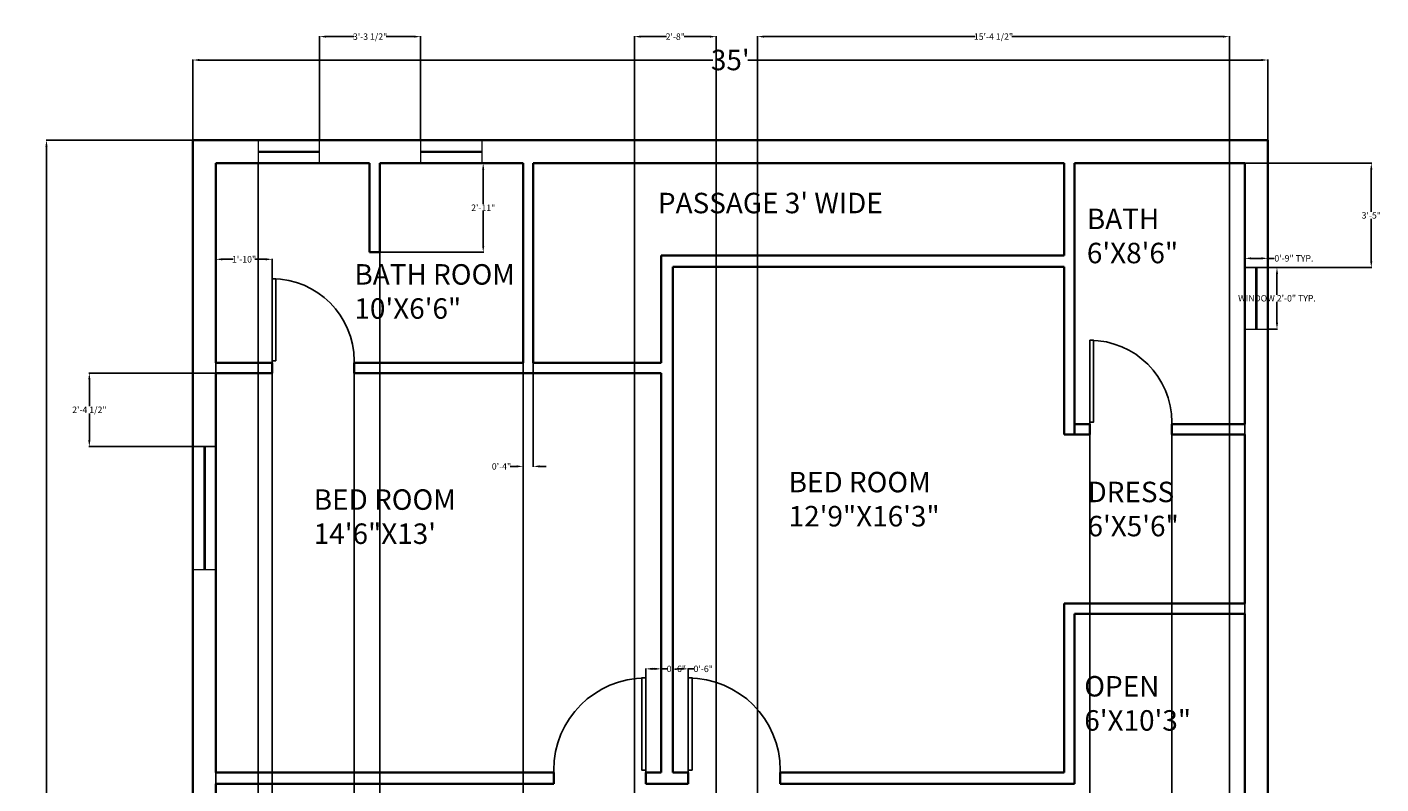
# Model space of a CAD drawing. Units: inches. Extents: x 1737 to 2270, y 2551 to 3419.
# Tile 4 of 4: x 1737 to 2266, y 3124 to 3419. Entities that reach past the tile are written whole.
import ezdxf

# ---------------------------------------------------------------- set-up
doc = ezdxf.new("R2010")
doc.units = ezdxf.units.IN
doc.header["$MEASUREMENT"] = 0
doc.layers.get('0').update_dxf_attribs({"color": 60})
for name, color, linetype, lineweight in [('A-ANNO-DIMS', 2, 'Continuous', 18), ('A-AREA-IDEN', 231, 'Continuous', 18), ('DOOR', 20, 'Continuous', 25), ('WALL', 60, 'Continuous', 35), ('WINDOW', 30, 'Continuous', 18)]:
    doc.layers.add(name, color=color, linetype=linetype, lineweight=lineweight)
doc.styles.get("Standard").update_dxf_attribs({"font": 'arial.ttf'})
doc.dimstyles.get("Standard").update_dxf_attribs({"dimtxt": 2.5, "dimasz": 2.5, "dimexe": 0.18, "dimexo": 0.0625, "dimgap": 0.09, "dimtad": 0, "dimtih": 1, "dimtoh": 1, "dimzin": 0, "dimdsep": 46, "dimlunit": 3, "dimtxsty": 'Standard', "dimcen": 0.09, "dimadec": 0, "dimazin": 0, "dimtfac": 1, "dimtofl": 0, "dimtmove": 0, "dimatfit": 3, "dimfxl": 1, "dimtolj": 1, "dimtzin": 0, "dimarcsym": 0})

# ---------------------------------------------------------------- blocks, each defined once
blk = doc.blocks.new('*U2')
for p, q in [((0, 0), (0, -6)), ((40, 0), (40, -6))]:
    blk.add_line(p, q)
blk.add_lwpolyline([(0, 0), (0, 40), (1.75, 40), (1.75, 0)], close=True)
blk.add_arc((0, 0), 40, 0, 90)
blk = doc.blocks.new('*D5')
at = {"layer": 'A-ANNO-DIMS', "color": 0, "lineweight": -2, "transparency": 16777216}
for p, q in [((1802.15, 3375.16), (1744.83, 3375.16)), ((1745.01, 3372.66), (1745.01, 2989.33)), ((1745.01, 2597.66), (1745.01, 2980.98)), ((1802.15, 2595.16), (1744.83, 2595.16))]:
    blk.add_line(p, q, dxfattribs=at)
at = {"layer": 'A-ANNO-DIMS', "color": 0, "transparency": 16777216}
for points in [[(1744.59, 3372.66), (1745.42, 3372.66), (1745.01, 3375.16)], [(1744.59, 2597.66), (1745.42, 2597.66), (1745.01, 2595.16)]]:
    blk.add_solid(points, dxfattribs=at)
at = {"layer": 'Defpoints', "color": 0, "transparency": 16777216}
for p in [(1802.21, 3375.16), (1745.01, 2595.16), (1802.21, 2595.16)]:
    blk.add_point(p, dxfattribs=at)
at = {"layer": 'A-ANNO-DIMS', "color": 0, "transparency": 16777216, "insert": (1745.01, 2985.16), "char_height": 8, "attachment_point": 5}
blk.add_mtext("\\A1;65'", dxfattribs=at)
blk = doc.blocks.new('*D6')
at = {"layer": 'A-ANNO-DIMS', "color": 0, "lineweight": -2, "transparency": 16777216}
for p, q in [((1802.21, 3375.22), (1802.21, 3406.65)), ((1804.71, 3406.47), (2005.33, 3406.47)), ((2219.71, 3406.47), (2019.08, 3406.47)), ((2222.21, 3375.22), (2222.21, 3406.65))]:
    blk.add_line(p, q, dxfattribs=at)
at = {"layer": 'A-ANNO-DIMS', "color": 0, "transparency": 16777216}
for points in [[(1804.71, 3406.88), (1804.71, 3406.05), (1802.21, 3406.47)], [(2219.71, 3406.88), (2219.71, 3406.05), (2222.21, 3406.47)]]:
    blk.add_solid(points, dxfattribs=at)
at = {"layer": 'Defpoints', "color": 0, "transparency": 16777216}
for p in [(2222.21, 3406.47), (1802.21, 3375.16), (2222.21, 3375.16)]:
    blk.add_point(p, dxfattribs=at)
at = {"layer": 'A-ANNO-DIMS', "color": 0, "transparency": 16777216, "insert": (2012.21, 3406.47), "char_height": 8, "attachment_point": 5}
blk.add_mtext("\\A1;35'", dxfattribs=at)
blk = doc.blocks.new('WIN-48IN')
for p, q in [((4.25, 48), (4.25, 0)), ((4.75, 48), (4.75, 0))]:
    blk.add_line(p, q)
blk.add_lwpolyline([(0, 48), (0, 0), (9, 0), (9, 48)], close=True)
blk = doc.blocks.new('WIN-24IN')
for p, q in [((0, 4.75), (24, 4.75)), ((0, 4.25), (24, 4.25))]:
    blk.add_line(p, q)
blk.add_lwpolyline([(0, 0), (24, 0), (24, 9), (0, 9)], close=True)
blk = doc.blocks.new('*D11')
at = {"layer": 'A-ANNO-DIMS', "color": 0, "lineweight": -2, "transparency": 16777216}
for p, q in [((2222.27, 3325.38), (2225.99, 3325.38)), ((2225.81, 3322.88), (2225.81, 3314.76)), ((2225.81, 3303.88), (2225.81, 3311.99)), ((2222.27, 3301.38), (2225.99, 3301.38))]:
    blk.add_line(p, q, dxfattribs=at)
at = {"layer": 'A-ANNO-DIMS', "color": 0, "transparency": 16777216}
for points in [[(2225.39, 3322.88), (2226.23, 3322.88), (2225.81, 3325.38)], [(2225.39, 3303.88), (2226.23, 3303.88), (2225.81, 3301.38)]]:
    blk.add_solid(points, dxfattribs=at)
at = {"layer": 'Defpoints', "color": 0, "transparency": 16777216}
for p in [(2222.21, 3325.38), (2222.21, 3301.38), (2225.81, 3301.38)]:
    blk.add_point(p, dxfattribs=at)
at = {"layer": 'A-ANNO-DIMS', "color": 0, "transparency": 16777216, "insert": (2225.81, 3313.38), "char_height": 2.5, "attachment_point": 5}
blk.add_mtext('\\A1;WINDOW 2\'-0" TYP.', dxfattribs=at)
blk = doc.blocks.new('*D12')
at = {"layer": 'A-ANNO-DIMS', "color": 0, "lineweight": -2, "transparency": 16777216}
for p, q in [((2213.21, 3325.44), (2213.21, 3329.16)), ((2215.71, 3328.98), (2219.71, 3328.98)), ((2222.21, 3325.44), (2222.21, 3329.16)), ((2222.21, 3328.98), (2224.71, 3328.98))]:
    blk.add_line(p, q, dxfattribs=at)
at = {"layer": 'A-ANNO-DIMS', "color": 0, "transparency": 16777216}
for points in [[(2215.71, 3329.39), (2215.71, 3328.56), (2213.21, 3328.98)], [(2219.71, 3329.39), (2219.71, 3328.56), (2222.21, 3328.98)]]:
    blk.add_solid(points, dxfattribs=at)
at = {"layer": 'Defpoints', "color": 0, "transparency": 16777216}
for p in [(2222.21, 3328.98), (2213.21, 3325.38), (2222.21, 3325.38)]:
    blk.add_point(p, dxfattribs=at)
at = {"layer": 'A-ANNO-DIMS', "color": 0, "transparency": 16777216, "insert": (2232.42, 3328.98), "char_height": 2.5, "attachment_point": 5}
blk.add_mtext('\\A1;0\'-9" TYP.', dxfattribs=at)
blk = doc.blocks.new('*D15')
at = {"layer": 'A-ANNO-DIMS', "color": 0, "lineweight": -2, "transparency": 16777216}
for p, q in [((1811.15, 3284.16), (1761.58, 3284.16)), ((1761.76, 3281.66), (1761.76, 3271.2)), ((1761.76, 3257.98), (1761.76, 3268.43)), ((1811.15, 3255.48), (1761.58, 3255.48))]:
    blk.add_line(p, q, dxfattribs=at)
at = {"layer": 'A-ANNO-DIMS', "color": 0, "transparency": 16777216}
for points in [[(1761.34, 3281.66), (1762.18, 3281.66), (1761.76, 3284.16)], [(1761.34, 3257.98), (1762.18, 3257.98), (1761.76, 3255.48)]]:
    blk.add_solid(points, dxfattribs=at)
at = {"layer": 'Defpoints', "color": 0, "transparency": 16777216}
for p in [(1811.21, 3284.16), (1761.76, 3255.48), (1811.21, 3255.48)]:
    blk.add_point(p, dxfattribs=at)
at = {"layer": 'A-ANNO-DIMS', "color": 0, "transparency": 16777216, "insert": (1761.76, 3269.82), "char_height": 2.5, "attachment_point": 5}
blk.add_mtext('\\A1;2\'-4 1/2"', dxfattribs=at)
blk = doc.blocks.new('*D17')
at = {"layer": 'A-ANNO-DIMS', "color": 0, "lineweight": -2, "transparency": 16777216}
for p, q in [((2213.27, 3366.16), (2262.84, 3366.16)), ((2262.66, 3363.66), (2262.66, 3347.13)), ((2262.66, 3327.88), (2262.66, 3344.4)), ((2213.27, 3325.38), (2262.84, 3325.38))]:
    blk.add_line(p, q, dxfattribs=at)
at = {"layer": 'A-ANNO-DIMS', "color": 0, "transparency": 16777216}
for points in [[(2262.24, 3363.66), (2263.08, 3363.66), (2262.66, 3366.16)], [(2262.24, 3327.88), (2263.08, 3327.88), (2262.66, 3325.38)]]:
    blk.add_solid(points, dxfattribs=at)
at = {"layer": 'Defpoints', "color": 0, "transparency": 16777216}
for p in [(2213.21, 3366.16), (2213.21, 3325.38), (2262.66, 3325.38)]:
    blk.add_point(p, dxfattribs=at)
at = {"layer": 'A-ANNO-DIMS', "color": 0, "transparency": 16777216, "insert": (2262.66, 3345.77), "char_height": 2.5, "attachment_point": 5}
blk.add_mtext('\\A1;3\'-5"', dxfattribs=at)
blk = doc.blocks.new('*D18')
at = {"layer": 'A-ANNO-DIMS', "color": 0, "lineweight": -2, "transparency": 16777216}
for p, q in [((1811.21, 3366.1), (1811.21, 2554.53)), ((1827.73, 3366.1), (1827.73, 2554.53)), ((1808.71, 2554.71), (1806.21, 2554.71)), ((1830.23, 2554.71), (1832.73, 2554.71))]:
    blk.add_line(p, q, dxfattribs=at)
at = {"layer": 'A-ANNO-DIMS', "color": 0, "transparency": 16777216}
for points in [[(1808.71, 2555.12), (1808.71, 2554.29), (1811.21, 2554.71)], [(1830.23, 2555.12), (1830.23, 2554.29), (1827.73, 2554.71)]]:
    blk.add_solid(points, dxfattribs=at)
at = {"layer": 'Defpoints', "color": 0, "transparency": 16777216}
for p in [(1811.21, 3366.16), (1827.73, 3366.16), (1827.73, 2554.71)]:
    blk.add_point(p, dxfattribs=at)
at = {"layer": 'A-ANNO-DIMS', "color": 0, "transparency": 16777216, "insert": (1819.47, 2554.71), "char_height": 2.5, "attachment_point": 5}
blk.add_mtext('\\A1;1\'-4 1/2"', dxfattribs=at)
blk = doc.blocks.new('*D19')
at = {"layer": 'A-ANNO-DIMS', "color": 0, "lineweight": -2, "transparency": 16777216}
for p, q in [((1851.73, 3375.22), (1851.73, 3415.79)), ((1854.23, 3415.61), (1865.13, 3415.61)), ((1888.69, 3415.61), (1877.78, 3415.61)), ((1891.19, 3375.22), (1891.19, 3415.79))]:
    blk.add_line(p, q, dxfattribs=at)
at = {"layer": 'A-ANNO-DIMS', "color": 0, "transparency": 16777216}
for points in [[(1854.23, 3416.02), (1854.23, 3415.19), (1851.73, 3415.61)], [(1888.69, 3416.02), (1888.69, 3415.19), (1891.19, 3415.61)]]:
    blk.add_solid(points, dxfattribs=at)
at = {"layer": 'Defpoints', "color": 0, "transparency": 16777216}
for p in [(1891.19, 3415.61), (1851.73, 3375.16), (1891.19, 3375.16)]:
    blk.add_point(p, dxfattribs=at)
at = {"layer": 'A-ANNO-DIMS', "color": 0, "transparency": 16777216, "insert": (1871.46, 3415.61), "char_height": 2.5, "attachment_point": 5}
blk.add_mtext('\\A1;3\'-3 1/2"', dxfattribs=at)
blk = doc.blocks.new('*D20')
at = {"layer": 'A-ANNO-DIMS', "color": 0, "lineweight": -2, "transparency": 16777216}
for p, q in [((2022.87, 2595.22), (2022.87, 3415.79)), ((2025.37, 3415.61), (2107.86, 3415.61)), ((2204.71, 3415.61), (2122.22, 3415.61)), ((2207.21, 2595.22), (2207.21, 3415.79))]:
    blk.add_line(p, q, dxfattribs=at)
at = {"layer": 'A-ANNO-DIMS', "color": 0, "transparency": 16777216}
for points in [[(2025.37, 3416.02), (2025.37, 3415.19), (2022.87, 3415.61)], [(2204.71, 3416.02), (2204.71, 3415.19), (2207.21, 3415.61)]]:
    blk.add_solid(points, dxfattribs=at)
at = {"layer": 'Defpoints', "color": 0, "transparency": 16777216}
for p in [(2207.21, 3415.61), (2022.87, 2595.16), (2207.21, 2595.16)]:
    blk.add_point(p, dxfattribs=at)
at = {"layer": 'A-ANNO-DIMS', "color": 0, "transparency": 16777216, "insert": (2115.04, 3415.61), "char_height": 2.5, "attachment_point": 5}
blk.add_mtext('\\A1;15\'-4 1/2"', dxfattribs=at)
blk = doc.blocks.new('*D24')
at = {"layer": 'A-ANNO-DIMS', "color": 0, "lineweight": -2, "transparency": 16777216}
for p, q in [((1833.21, 3284.1), (1833.21, 2554.53)), ((1865.21, 3284.1), (1865.21, 2554.53)), ((1835.71, 2554.71), (1845.77, 2554.71)), ((1862.71, 2554.71), (1852.64, 2554.71))]:
    blk.add_line(p, q, dxfattribs=at)
at = {"layer": 'A-ANNO-DIMS', "color": 0, "transparency": 16777216}
for points in [[(1835.71, 2555.12), (1835.71, 2554.29), (1833.21, 2554.71)], [(1862.71, 2555.12), (1862.71, 2554.29), (1865.21, 2554.71)]]:
    blk.add_solid(points, dxfattribs=at)
at = {"layer": 'Defpoints', "color": 0, "transparency": 16777216}
for p in [(1833.21, 3284.16), (1865.21, 3284.16), (1865.21, 2554.71)]:
    blk.add_point(p, dxfattribs=at)
at = {"layer": 'A-ANNO-DIMS', "color": 0, "transparency": 16777216, "insert": (1849.21, 2554.71), "char_height": 2.5, "attachment_point": 5}
blk.add_mtext('\\A1;2\'-8"', dxfattribs=at)
blk = doc.blocks.new('*D29')
at = {"layer": 'A-ANNO-DIMS', "color": 0, "lineweight": -2, "transparency": 16777216}
for p, q in [((1974.71, 2758.72), (1974.71, 3415.79)), ((1977.21, 3415.61), (1987.27, 3415.61)), ((2004.21, 3415.61), (1994.14, 3415.61)), ((2006.71, 2758.72), (2006.71, 3415.79))]:
    blk.add_line(p, q, dxfattribs=at)
at = {"layer": 'A-ANNO-DIMS', "color": 0, "transparency": 16777216}
for points in [[(1977.21, 3416.02), (1977.21, 3415.19), (1974.71, 3415.61)], [(2004.21, 3416.02), (2004.21, 3415.19), (2006.71, 3415.61)]]:
    blk.add_solid(points, dxfattribs=at)
at = {"layer": 'Defpoints', "color": 0, "transparency": 16777216}
for p in [(2006.71, 3415.61), (1974.71, 2758.66), (2006.71, 2758.66)]:
    blk.add_point(p, dxfattribs=at)
at = {"layer": 'A-ANNO-DIMS', "color": 0, "transparency": 16777216, "insert": (1990.71, 3415.61), "char_height": 2.5, "attachment_point": 5}
blk.add_mtext('\\A1;2\'-8"', dxfattribs=at)
blk = doc.blocks.new('*D33')
at = {"layer": 'A-ANNO-DIMS', "color": 0, "lineweight": -2, "transparency": 16777216}
for p, q in [((1811.21, 3288.22), (1811.21, 3328.79)), ((1813.71, 3328.61), (1817.94, 3328.61)), ((1830.71, 3328.61), (1826.48, 3328.61)), ((1833.21, 3288.22), (1833.21, 3328.79))]:
    blk.add_line(p, q, dxfattribs=at)
at = {"layer": 'A-ANNO-DIMS', "color": 0, "transparency": 16777216}
for points in [[(1813.71, 3329.02), (1813.71, 3328.19), (1811.21, 3328.61)], [(1830.71, 3329.02), (1830.71, 3328.19), (1833.21, 3328.61)]]:
    blk.add_solid(points, dxfattribs=at)
at = {"layer": 'Defpoints', "color": 0, "transparency": 16777216}
for p in [(1833.21, 3328.61), (1811.21, 3288.16), (1833.21, 3288.16)]:
    blk.add_point(p, dxfattribs=at)
at = {"layer": 'A-ANNO-DIMS', "color": 0, "transparency": 16777216, "insert": (1822.21, 3328.61), "char_height": 2.5, "attachment_point": 5}
blk.add_mtext('\\A1;1\'-10"', dxfattribs=at)
blk = doc.blocks.new('*D36')
at = {"layer": 'A-ANNO-DIMS', "color": 0, "lineweight": -2, "transparency": 16777216}
for p, q in [((2152.71, 3260.1), (2152.71, 2554.53)), ((2184.71, 3260.1), (2184.71, 2554.53)), ((2155.21, 2554.71), (2165.27, 2554.71)), ((2182.21, 2554.71), (2172.14, 2554.71))]:
    blk.add_line(p, q, dxfattribs=at)
at = {"layer": 'A-ANNO-DIMS', "color": 0, "transparency": 16777216}
for points in [[(2155.21, 2555.12), (2155.21, 2554.29), (2152.71, 2554.71)], [(2182.21, 2555.12), (2182.21, 2554.29), (2184.71, 2554.71)]]:
    blk.add_solid(points, dxfattribs=at)
at = {"layer": 'Defpoints', "color": 0, "transparency": 16777216}
for p in [(2152.71, 3260.16), (2184.71, 3260.16), (2184.71, 2554.71)]:
    blk.add_point(p, dxfattribs=at)
at = {"layer": 'A-ANNO-DIMS', "color": 0, "transparency": 16777216, "insert": (2168.71, 2554.71), "char_height": 2.5, "attachment_point": 5}
blk.add_mtext('\\A1;2\'-8"', dxfattribs=at)
blk = doc.blocks.new('*D38')
at = {"layer": 'A-ANNO-DIMS', "color": 0, "lineweight": -2, "transparency": 16777216}
for p, q in [((1875.27, 3366.16), (1915.84, 3366.16)), ((1915.66, 3363.66), (1915.66, 3350.1)), ((1915.66, 3333.86), (1915.66, 3347.41)), ((1875.27, 3331.36), (1915.84, 3331.36))]:
    blk.add_line(p, q, dxfattribs=at)
at = {"layer": 'A-ANNO-DIMS', "color": 0, "transparency": 16777216}
for points in [[(1915.24, 3363.66), (1916.08, 3363.66), (1915.66, 3366.16)], [(1915.24, 3333.86), (1916.08, 3333.86), (1915.66, 3331.36)]]:
    blk.add_solid(points, dxfattribs=at)
at = {"layer": 'Defpoints', "color": 0, "transparency": 16777216}
for p in [(1875.21, 3366.16), (1875.21, 3331.36), (1915.66, 3331.36)]:
    blk.add_point(p, dxfattribs=at)
at = {"layer": 'A-ANNO-DIMS', "color": 0, "transparency": 16777216, "insert": (1915.66, 3348.76), "char_height": 2.5, "attachment_point": 5}
blk.add_mtext('\\A1;2\'-11"', dxfattribs=at)
blk = doc.blocks.new('*D39')
at = {"layer": 'A-ANNO-DIMS', "color": 0, "lineweight": -2, "transparency": 16777216}
for p, q in [((1875.21, 3366.1), (1875.21, 2554.53)), ((1931.21, 3366.1), (1931.21, 2554.53)), ((1877.71, 2554.71), (1899.75, 2554.71)), ((1928.71, 2554.71), (1906.67, 2554.71))]:
    blk.add_line(p, q, dxfattribs=at)
at = {"layer": 'A-ANNO-DIMS', "color": 0, "transparency": 16777216}
for points in [[(1877.71, 2555.12), (1877.71, 2554.29), (1875.21, 2554.71)], [(1928.71, 2555.12), (1928.71, 2554.29), (1931.21, 2554.71)]]:
    blk.add_solid(points, dxfattribs=at)
at = {"layer": 'Defpoints', "color": 0, "transparency": 16777216}
for p in [(1875.21, 3366.16), (1931.21, 3366.16), (1931.21, 2554.71)]:
    blk.add_point(p, dxfattribs=at)
at = {"layer": 'A-ANNO-DIMS', "color": 0, "transparency": 16777216, "insert": (1903.21, 2554.71), "char_height": 2.5, "attachment_point": 5}
blk.add_mtext('\\A1;4\'-8"', dxfattribs=at)
blk = doc.blocks.new('*D40')
at = {"layer": 'A-ANNO-DIMS', "color": 0, "lineweight": -2, "transparency": 16777216}
for p, q in [((1979.21, 3128.22), (1979.21, 3168.79)), ((1985.21, 3128.22), (1985.21, 3168.79)), ((1981.71, 3168.61), (1982.71, 3168.61)), ((1985.21, 3168.61), (1987.71, 3168.61))]:
    blk.add_line(p, q, dxfattribs=at)
at = {"layer": 'A-ANNO-DIMS', "color": 0, "transparency": 16777216}
for points in [[(1981.71, 3169.02), (1981.71, 3168.19), (1979.21, 3168.61)], [(1982.71, 3169.02), (1982.71, 3168.19), (1985.21, 3168.61)]]:
    blk.add_solid(points, dxfattribs=at)
at = {"layer": 'Defpoints', "color": 0, "transparency": 16777216}
for p in [(1985.21, 3168.61), (1979.21, 3128.16), (1985.21, 3128.16)]:
    blk.add_point(p, dxfattribs=at)
at = {"layer": 'A-ANNO-DIMS', "color": 0, "transparency": 16777216, "insert": (1991.12, 3168.61), "char_height": 2.5, "attachment_point": 5}
blk.add_mtext('\\A1;0\'-6"', dxfattribs=at)
blk = doc.blocks.new('*D41')
at = {"layer": 'A-ANNO-DIMS', "color": 0, "lineweight": -2, "transparency": 16777216}
for p, q in [((1989.71, 3128.22), (1989.71, 3168.79)), ((1995.71, 3128.22), (1995.71, 3168.79)), ((1992.21, 3168.61), (1993.21, 3168.61)), ((1995.71, 3168.61), (1998.21, 3168.61))]:
    blk.add_line(p, q, dxfattribs=at)
at = {"layer": 'A-ANNO-DIMS', "color": 0, "transparency": 16777216}
for points in [[(1992.21, 3169.02), (1992.21, 3168.19), (1989.71, 3168.61)], [(1993.21, 3169.02), (1993.21, 3168.19), (1995.71, 3168.61)]]:
    blk.add_solid(points, dxfattribs=at)
at = {"layer": 'Defpoints', "color": 0, "transparency": 16777216}
for p in [(1995.71, 3168.61), (1989.71, 3128.16), (1995.71, 3128.16)]:
    blk.add_point(p, dxfattribs=at)
at = {"layer": 'A-ANNO-DIMS', "color": 0, "transparency": 16777216, "insert": (2001.62, 3168.61), "char_height": 2.5, "attachment_point": 5}
blk.add_mtext('\\A1;0\'-6"', dxfattribs=at)
blk = doc.blocks.new('*D42')
at = {"layer": 'A-ANNO-DIMS', "color": 0, "lineweight": -2, "transparency": 16777216}
for p, q in [((2213.21, 3264.1), (2213.21, 2554.53)), ((2184.71, 3263.5), (2184.71, 2554.53)), ((2187.21, 2554.71), (2192.61, 2554.71)), ((2210.71, 2554.71), (2205.31, 2554.71))]:
    blk.add_line(p, q, dxfattribs=at)
at = {"layer": 'A-ANNO-DIMS', "color": 0, "transparency": 16777216}
for points in [[(2187.21, 2555.12), (2187.21, 2554.29), (2184.71, 2554.71)], [(2210.71, 2555.12), (2210.71, 2554.29), (2213.21, 2554.71)]]:
    blk.add_solid(points, dxfattribs=at)
at = {"layer": 'Defpoints', "color": 0, "transparency": 16777216}
for p in [(2213.21, 3264.16), (2184.71, 3263.56), (2213.21, 2554.71)]:
    blk.add_point(p, dxfattribs=at)
at = {"layer": 'A-ANNO-DIMS', "color": 0, "transparency": 16777216, "insert": (2198.96, 2554.71), "char_height": 2.5, "attachment_point": 5}
blk.add_mtext('\\A1;2\'-4 1/2"', dxfattribs=at)
blk = doc.blocks.new('*D52')
at = {"layer": 'A-ANNO-DIMS', "color": 0, "lineweight": -2, "transparency": 16777216}
for p, q in [((1931.21, 3288.1), (1931.21, 3247.53)), ((1935.21, 3288.1), (1935.21, 3247.53)), ((1928.71, 3247.71), (1926.21, 3247.71)), ((1937.71, 3247.71), (1940.21, 3247.71))]:
    blk.add_line(p, q, dxfattribs=at)
at = {"layer": 'A-ANNO-DIMS', "color": 0, "transparency": 16777216}
for points in [[(1928.71, 3248.12), (1928.71, 3247.29), (1931.21, 3247.71)], [(1937.71, 3248.12), (1937.71, 3247.29), (1935.21, 3247.71)]]:
    blk.add_solid(points, dxfattribs=at)
at = {"layer": 'Defpoints', "color": 0, "transparency": 16777216}
for p in [(1931.21, 3288.16), (1935.21, 3288.16), (1931.21, 3247.71)]:
    blk.add_point(p, dxfattribs=at)
at = {"layer": 'A-ANNO-DIMS', "color": 0, "transparency": 16777216, "insert": (1922.8, 3247.71), "char_height": 2.5, "attachment_point": 5}
blk.add_mtext('\\A1;0\'-4"', dxfattribs=at)

msp = doc.modelspace()

# ---------------------------------------------------------------- linework, layer by layer
at = {"layer": 'WALL'}
for p, q in [((2222.209, 3375.158), (1802.209, 3375.158)), ((1802.209, 3375.158), (1802.209, 2669.158)), ((2222.209, 2595.158), (2222.209, 3375.158)), ((1811.209, 3366.158), (1811.209, 3288.158)), ((1871.209, 3366.158), (1811.209, 3366.158)), ((1871.209, 3366.158), (1871.209, 3331.355)), ((1875.209, 3366.158), (1875.209, 3331.355)), ((1931.209, 3366.158), (1875.209, 3366.158)), ((1931.209, 3366.158), (1931.209, 3288.158)), ((2142.709, 3366.158), (1935.209, 3366.158)), ((1935.209, 3366.158), (1935.209, 3288.158)), ((2142.709, 3366.158), (2142.709, 3330.158)), ((2213.209, 3366.158), (2146.709, 3366.158)), ((2146.709, 3366.158), (2146.709, 3260.158)), ((2213.209, 3264.158), (2213.209, 3366.158)), ((1871.209, 3331.355), (1875.209, 3331.355)), ((1985.209, 3330.158), (1985.209, 3288.158)), ((2142.709, 3330.158), (1985.209, 3330.158)), ((1989.709, 3325.658), (1989.709, 3128.158)), ((2142.709, 3325.658), (1989.709, 3325.658)), ((2142.709, 3325.658), (2142.709, 3260.158)), ((2142.709, 3325.658), (2142.709, 3288.158)), ((1833.209, 3288.158), (1811.209, 3288.158)), ((1833.209, 3288.158), (1833.209, 3284.158)), ((1865.209, 3288.158), (1865.209, 3284.158)), ((1931.209, 3288.158), (1865.209, 3288.158)), ((1871.209, 3288.158), (1865.209, 3288.158)), ((1985.209, 3288.158), (1935.209, 3288.158)), ((1811.209, 3284.158), (1811.209, 3128.158)), ((1833.209, 3284.158), (1811.209, 3284.158)), ((1985.209, 3284.158), (1865.209, 3284.158)), ((1985.209, 3284.158), (1985.209, 3128.158)), ((2152.709, 3264.158), (2146.709, 3264.158)), ((2152.709, 3264.158), (2152.709, 3260.158)), ((2213.209, 3264.158), (2184.709, 3264.158)), ((2184.709, 3264.158), (2184.709, 3260.158)), ((2146.709, 3260.158), (2142.709, 3260.158)), ((2152.709, 3260.158), (2146.709, 3260.158)), ((2213.209, 3260.158), (2184.709, 3260.158)), ((2213.209, 3194.158), (2213.209, 3260.158)), ((2146.709, 3194.158), (2142.709, 3194.158)), ((2142.709, 3194.158), (2142.709, 3128.158)), ((2213.209, 3194.158), (2146.709, 3194.158)), ((2213.209, 3190.158), (2146.709, 3190.158)), ((2146.709, 3190.158), (2146.709, 3123.658)), ((2213.209, 3070.658), (2213.209, 3190.158)), ((1943.209, 3128.158), (1811.209, 3128.158)), ((1943.209, 3128.158), (1943.209, 3123.658)), ((1979.209, 3128.158), (1979.209, 3123.658)), ((1985.209, 3128.158), (1979.209, 3128.158)), ((1995.709, 3128.158), (1989.709, 3128.158)), ((1995.709, 3128.158), (1995.709, 3123.658)), ((2142.709, 3128.158), (2031.709, 3128.158)), ((2031.709, 3128.158), (2031.709, 3123.658)), ((1811.209, 3123.658), (1811.209, 2934.658)), ((1943.209, 3123.658), (1811.209, 3123.658)), ((1995.709, 3123.658), (1979.209, 3123.658)), ((2060.209, 3123.658), (2031.709, 3123.658)), ((2060.209, 3123.658), (2064.709, 3123.658)), ((2146.709, 3123.658), (2064.709, 3123.658))]:
    msp.add_line(p, q, dxfattribs=at)

# ---------------------------------------------------------------- block references
at = {"layer": 'DOOR'}
for p, xscale, yscale, zscale in [((1833.209, 3288.958), 0.7999999999999955, 0.7999999999999955, 0.7999999999999955), ((2152.709, 3264.958), 0.8, 0.8, 0.8), ((1979.209, 3129.058), -0.8999999999999948, 0.8999999999999948, 0.8999999999999948), ((1995.709, 3129.058), 0.8999999999999948, 0.8999999999999948, 0.8999999999999948)]:
    msp.add_blockref('*U2', p, dxfattribs=dict(at, xscale=xscale, yscale=yscale, zscale=zscale))
at = {"layer": 'WINDOW'}
for name, p in [('WIN-24IN', (1827.725, 3366.158)), ('WIN-24IN', (1891.19, 3366.158)), ('WIN-48IN', (1802.209, 3207.476))]:
    msp.add_blockref(name, p, dxfattribs=at)
at = {"layer": 'WINDOW', "rotation": 270.0000000000033}
msp.add_blockref('WIN-24IN', (2213.209, 3325.377), dxfattribs=at)

# ---------------------------------------------------------------- texts
at = {"layer": 'A-AREA-IDEN', "char_height": 8, "attachment_point": 1}
for s, width, insert in [("\\pxt7;PASSAGE 3' WIDE", 108.6641, (1983.923, 3354.596)), ('BATH\\P6\'X8\'6"', 60.91246, (2151.525, 3348.403)), ('BATH ROOM\\P10\'X6\'6"', 70.74426, (1865.334, 3326.713)), ('BED ROOM\\P12\'9"X16\'3"', 60.91246, (2035.007, 3245.581)), ('BED ROOM\\P14\'6"X13\'', 60.91246, (1849.445, 3238.745)), ('DRESS\\P6\'X5\'6"', 60.91246, (2151.774, 3241.724)), ('OPEN\\P6\'X10\'3"', 60.91246, (2150.519, 3165.803))]:
    msp.add_mtext_dynamic_manual_height_columns(s, width=width, gutter_width=1, heights=[0], dxfattribs=dict(at, insert=insert))

# ---------------------------------------------------------------- dimensions: what is measured, and where the dimension line sits
at = {"layer": 'A-ANNO-DIMS'}
for base, p1, p2, picture, middle in [((1891.19, 3415.608), (1851.725, 3375.158), (1891.19, 3375.158), '*D19', (1871.458, 3415.608)), ((2207.209, 3415.608), (2022.872, 2595.158), (2207.209, 2595.158), '*D20', (2115.041, 3415.608)), ((2006.709, 3415.608), (1974.709, 2758.658), (2006.709, 2758.658), '*D29', (1990.709, 3415.608)), ((1827.725, 2554.708), (1811.209, 3366.158), (1827.725, 3366.158), '*D18', (1819.467, 2554.708)), ((1931.209, 2554.708), (1875.209, 3366.158), (1931.209, 3366.158), '*D39', (1903.209, 2554.708)), ((1833.209, 3328.608), (1811.209, 3288.158), (1833.209, 3288.158), '*D33', (1822.209, 3328.608)), ((1865.209, 2554.708), (1833.209, 3284.158), (1865.209, 3284.158), '*D24', (1849.209, 2554.708)), ((2213.209, 2554.708), (2184.709, 3263.558), (2213.209, 3264.158), '*D42', (2198.959, 2554.708)), ((2184.709, 2554.708), (2152.709, 3260.158), (2184.709, 3260.158), '*D36', (2168.709, 2554.708)), ((1985.209, 3168.608), (1979.209, 3128.158), (1985.209, 3128.158), '*D40', (1991.122, 3168.608)), ((1995.709, 3168.608), (1989.709, 3128.158), (1995.709, 3128.158), '*D41', (2001.622, 3168.608))]:
    dim = msp.add_linear_dim(base=base, p1=p1, p2=p2, dimstyle='Standard', override={"dimdec": 1, "dimlfac": 1, "dimrnd": 0, "dimzin": 1, "dimdsep": 46, "dimlunit": 4, "dimfrac": 2}, dxfattribs=at)
    dim.commit()
    dim.dimension.update_dxf_attribs({"geometry": picture, "text_midpoint": middle})
for p2, distance, picture, middle in [((2222.209, 3375.158), 31.31, '*D6', (2012.209, 3406.468)), ((1802.209, 2595.158), -57.201, '*D5', (1745.008, 2985.158))]:
    dim = msp.add_aligned_dim(p1=(1802.209, 3375.158), p2=p2, distance=distance, dimstyle='Standard', override={"dimtxt": 8, "dimclrd": 0, "dimclre": 0, "dimclrt": 0}, dxfattribs=at)
    dim.commit()
    dim.dimension.update_dxf_attribs({"geometry": picture, "text_midpoint": middle})
for base, p1, p2, angle, picture, middle in [((1915.659, 3331.355), (1875.209, 3366.158), (1875.209, 3331.355), 270, '*D38', (1915.659, 3348.757)), ((2262.659, 3325.377), (2213.209, 3366.158), (2213.209, 3325.377), 90, '*D17', (2262.659, 3345.768)), ((1931.209, 3247.708), (1935.209, 3288.158), (1931.209, 3288.158), 180, '*D52', (1922.796, 3247.708)), ((1761.759, 3255.476), (1811.209, 3284.158), (1811.209, 3255.476), 90, '*D15', (1761.759, 3269.817))]:
    dim = msp.add_linear_dim(base=base, p1=p1, p2=p2, angle=angle, dimstyle='Standard', override={"dimdec": 1, "dimlfac": 1, "dimrnd": 0, "dimzin": 1, "dimdsep": 46, "dimlunit": 4, "dimfrac": 2}, dxfattribs=at)
    dim.commit()
    dim.dimension.update_dxf_attribs({"geometry": picture, "text_midpoint": middle})
for base, p1, p2, angle, text, picture, middle in [((2222.209, 3328.977), (2213.209, 3325.377), (2222.209, 3325.377), 0, '<> TYP.', '*D12', (2232.418, 3328.977)), ((2225.809, 3301.377), (2222.209, 3325.377), (2222.209, 3301.377), 270, 'WINDOW <> TYP.', '*D11', (2225.809, 3313.377))]:
    dim = msp.add_linear_dim(base=base, p1=p1, p2=p2, angle=angle, text=text, dimstyle='Standard', override={"dimdec": 1, "dimlfac": 1, "dimrnd": 0, "dimzin": 1, "dimdsep": 46, "dimlunit": 4, "dimfrac": 2}, dxfattribs=at)
    dim.commit()
    dim.dimension.update_dxf_attribs({"geometry": picture, "text_midpoint": middle})

doc.saveas('drawing.dxf')
